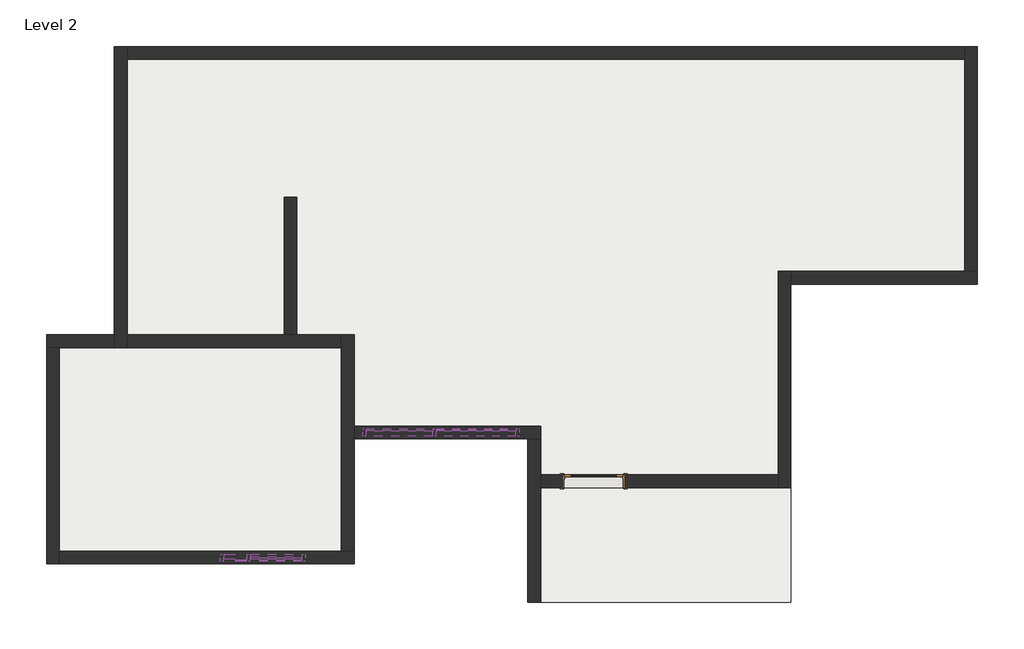
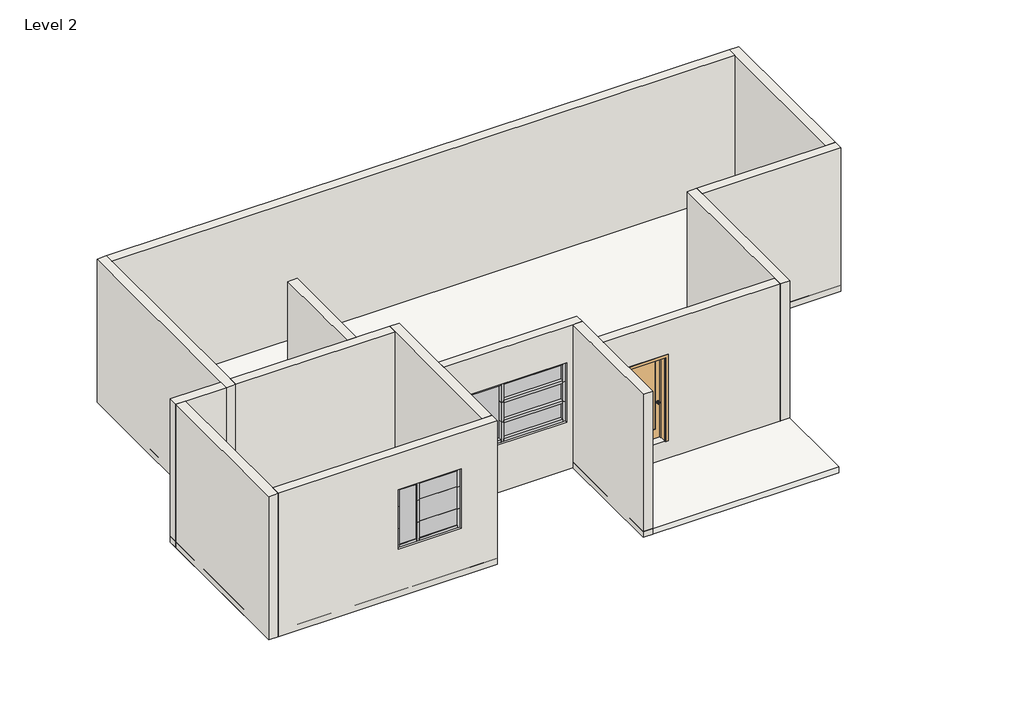
# One storey: 30 members, 14 walls, 8 plates, 1 door, 1 roof.
"""IFC4 building model written with IfcOpenShell, lengths in millimetres."""

from ifc_helpers import new_model, si_unit, frame, origin, place, context, project, spatial, polyline, outline, extrude, faceted_brep, transform, mapped, element, save
from components import door_0f538abb, member_df2e51ae, member_dc106669, member_ff82125d, member_323df77c, member_bc554fa6, member_86d06fe4, member_50cacee6, member_7fd687a9, member_26d67f61, member_e9c7f4a4, member_90750a43, member_6df10a9f, system_panel_glazed_08f033f8, system_panel_glazed_aa4e1581, system_panel_glazed_b16bc715, system_panel_glazed_e5754967, system_panel_glazed_03bb9a0f, system_panel_glazed_a826d7bb

model = new_model("IFC4")

# Units and contexts
model_context = context("Model", 3, world=origin())
ifc_project = project(units=[si_unit("LENGTHUNIT", "METRE", prefix="MILLI")], contexts=[model_context])

# Site, building, storey
site = spatial("IfcSite", under=ifc_project)
building = spatial("IfcBuilding", under=site)
storey = spatial("IfcBuildingStorey", under=building, Name="Level 2", Elevation=3048.0)

# Door
placement = place(None, origin())
door_shape = door_0f538abb(model_context)
element("IfcDoor", 1, ObjectType="Door-Interior-Single-1_Panel-Wood : 42\" x 84\"", at=placement, inside=storey, context=model_context, shape_type="MappedRepresentation", body=[
    mapped(door_shape, transform((-1951.8981007, 5916.5450124, 3657.6), x_axis=(-1.0, 0.0, 0.0), y_axis=(0.0, -1.0, 0.0), z_axis=(0.0, 0.0, 1.0))),
])

# Members
member_shape = member_df2e51ae(model_context)
element("IfcMember", 2, ObjectType="Rectangular Mullion : 1\" Square", at=placement, inside=storey, context=model_context, shape_type="MappedRepresentation", body=[
    mapped(member_shape, transform((-8117.7481007, 4541.7700124, 5308.6), x_axis=(0.0, 0.0, 1.0), y_axis=(0.0, 1.0, 0.0), z_axis=(-1.0, 0.0, 0.0))),
])
element("IfcMember", 3, ObjectType="Rectangular Mullion : 1\" Square", at=placement, inside=storey, context=model_context, shape_type="MappedRepresentation", body=[
    mapped(member_shape, transform((-8117.7481007, 4541.7700124, 4749.8), x_axis=(0.0, 0.0, 1.0), y_axis=(0.0, 1.0, 0.0), z_axis=(-1.0, 0.0, 0.0))),
])
member_2_shape = member_dc106669(model_context)
element("IfcMember", 4, ObjectType="Rectangular Mullion : 2.5\" x 5\" rectangular", at=placement, inside=storey, context=model_context, shape_type="MappedRepresentation", body=[
    mapped(member_2_shape, transform((-8593.9981007, 4541.7700124, 5791.2), x_axis=(0.0, 0.0, 1.0), y_axis=(0.0, 1.0, 0.0), z_axis=(-1.0, 0.0, 0.0))),
])
member_3_shape = member_ff82125d(model_context)
element("IfcMember", 5, ObjectType="Rectangular Mullion : 2.5\" x 5\" rectangular", at=placement, inside=storey, context=model_context, shape_type="MappedRepresentation", body=[
    mapped(member_3_shape, transform((-7196.9981007, 4541.7700124, 4267.2), x_axis=(0.0, 0.0, -1.0), y_axis=(0.0, 1.0, 0.0), z_axis=(1.0, 0.0, 0.0))),
])
member_4_shape = member_323df77c(model_context)
element("IfcMember", 6, ObjectType="Rectangular Mullion : 2.5\" x 5\" rectangular", at=placement, inside=storey, context=model_context, shape_type="MappedRepresentation", body=[
    mapped(member_4_shape, transform((-8149.4981007, 4541.7700124, 4267.2), x_axis=(-1.0, 0.0, 0.0), y_axis=(0.0, 1.0, 0.0), z_axis=(0.0, 0.0, -1.0))),
])
element("IfcMember", 7, ObjectType="Rectangular Mullion : 2.5\" x 5\" rectangular", at=placement, inside=storey, context=model_context, shape_type="MappedRepresentation", body=[
    mapped(member_2_shape, transform((-8181.2481007, 4541.7700124, 4267.2), x_axis=(0.0, 0.0, -1.0), y_axis=(0.0, 1.0, 0.0), z_axis=(1.0, 0.0, 0.0))),
])
element("IfcMember", 8, ObjectType="Rectangular Mullion : 2.5\" x 5\" rectangular", at=placement, inside=storey, context=model_context, shape_type="MappedRepresentation", body=[
    mapped(member_3_shape, transform((-8117.7481007, 4541.7700124, 5791.2), x_axis=(0.0, 0.0, 1.0), y_axis=(0.0, 1.0, 0.0), z_axis=(-1.0, 0.0, 0.0))),
])
member_5_shape = member_bc554fa6(model_context)
element("IfcMember", 9, ObjectType="Rectangular Mullion : 2.5\" x 5\" rectangular", at=placement, inside=storey, context=model_context, shape_type="MappedRepresentation", body=[
    mapped(member_5_shape, transform((-8149.4981007, 4541.7700124, 4749.8), x_axis=(-1.0, 0.0, 0.0), y_axis=(0.0, 1.0, 0.0), z_axis=(0.0, 0.0, -1.0))),
])
element("IfcMember", 10, ObjectType="Rectangular Mullion : 2.5\" x 5\" rectangular", at=placement, inside=storey, context=model_context, shape_type="MappedRepresentation", body=[
    mapped(member_4_shape, transform((-8149.4981007, 4541.7700124, 5308.6), x_axis=(-1.0, 0.0, 0.0), y_axis=(0.0, 1.0, 0.0), z_axis=(0.0, 0.0, -1.0))),
])
member_6_shape = member_86d06fe4(model_context)
element("IfcMember", 11, ObjectType="Rectangular Mullion : 2.5\" x 5\" rectangular", at=placement, inside=storey, context=model_context, shape_type="MappedRepresentation", body=[
    mapped(member_6_shape, transform((-7133.4981007, 4541.7700124, 5791.2), x_axis=(1.0, 0.0, 0.0), y_axis=(0.0, 1.0, 0.0), z_axis=(0.0, 0.0, 1.0))),
])
element("IfcMember", 12, ObjectType="Rectangular Mullion : 2.5\" x 5\" rectangular", at=placement, inside=storey, context=model_context, shape_type="MappedRepresentation", body=[
    mapped(member_6_shape, transform((-8657.4981007, 4541.7700124, 4267.2), x_axis=(-1.0, 0.0, 0.0), y_axis=(0.0, 1.0, 0.0), z_axis=(0.0, 0.0, -1.0))),
])
member_7_shape = member_50cacee6(model_context)
element("IfcMember", 13, ObjectType="Rectangular Mullion : 2.5\" x 5\" rectangular", at=placement, inside=storey, context=model_context, shape_type="MappedRepresentation", body=[
    mapped(member_7_shape, transform((-8657.4981007, 4541.7700124, 4749.8), x_axis=(-1.0, 0.0, 0.0), y_axis=(0.0, 1.0, 0.0), z_axis=(0.0, 0.0, -1.0))),
])
element("IfcMember", 14, ObjectType="Rectangular Mullion : 2.5\" x 5\" rectangular", at=placement, inside=storey, context=model_context, shape_type="MappedRepresentation", body=[
    mapped(member_6_shape, transform((-8657.4981007, 4541.7700124, 5308.6), x_axis=(-1.0, 0.0, 0.0), y_axis=(0.0, 1.0, 0.0), z_axis=(0.0, 0.0, -1.0))),
])
element("IfcMember", 15, ObjectType="Rectangular Mullion : 2.5\" x 5\" rectangular", at=placement, inside=storey, context=model_context, shape_type="MappedRepresentation", body=[
    mapped(member_6_shape, transform((-7133.4981007, 4541.7700124, 4749.8), x_axis=(1.0, 0.0, 0.0), y_axis=(0.0, 1.0, 0.0), z_axis=(0.0, 0.0, 1.0))),
])
element("IfcMember", 16, ObjectType="Rectangular Mullion : 2.5\" x 5\" rectangular", at=placement, inside=storey, context=model_context, shape_type="MappedRepresentation", body=[
    mapped(member_7_shape, transform((-7133.4981007, 4541.7700124, 5308.6), x_axis=(1.0, 0.0, 0.0), y_axis=(0.0, 1.0, 0.0), z_axis=(0.0, 0.0, 1.0))),
])
member_8_shape = member_7fd687a9(model_context)
element("IfcMember", 17, ObjectType="Rectangular Mullion : 2.5\" x 5\" rectangular", at=placement, inside=storey, context=model_context, shape_type="MappedRepresentation", body=[
    mapped(member_8_shape, transform((-6104.7981007, 6789.6700124, 5791.2), x_axis=(-1.0, 0.0, 0.0), y_axis=(0.0, -1.0, 0.0), z_axis=(0.0, 0.0, 1.0))),
])
element("IfcMember", 18, ObjectType="Rectangular Mullion : 2.5\" x 5\" rectangular", at=placement, inside=storey, context=model_context, shape_type="MappedRepresentation", body=[
    mapped(member_8_shape, transform((-6104.7981007, 6789.6700124, 5283.2), x_axis=(-1.0, 0.0, 0.0), y_axis=(0.0, -1.0, 0.0), z_axis=(0.0, 0.0, 1.0))),
])
element("IfcMember", 19, ObjectType="Rectangular Mullion : 2.5\" x 5\" rectangular", at=placement, inside=storey, context=model_context, shape_type="MappedRepresentation", body=[
    mapped(member_8_shape, transform((-6104.7981007, 6789.6700124, 4775.2), x_axis=(-1.0, 0.0, 0.0), y_axis=(0.0, -1.0, 0.0), z_axis=(0.0, 0.0, 1.0))),
])
member_9_shape = member_26d67f61(model_context)
element("IfcMember", 20, ObjectType="Rectangular Mullion : 2.5\" x 5\" rectangular", at=placement, inside=storey, context=model_context, shape_type="MappedRepresentation", body=[
    mapped(member_9_shape, transform((-3348.8981007, 6789.6700124, 5791.2), x_axis=(0.0, 0.0, 1.0), y_axis=(0.0, -1.0, 0.0), z_axis=(1.0, 0.0, 0.0))),
])
member_10_shape = member_e9c7f4a4(model_context)
element("IfcMember", 21, ObjectType="Rectangular Mullion : 2.5\" x 5\" rectangular", at=placement, inside=storey, context=model_context, shape_type="MappedRepresentation", body=[
    mapped(member_10_shape, transform((-6041.2981007, 6789.6700124, 4267.2), x_axis=(0.0, 0.0, -1.0), y_axis=(0.0, -1.0, 0.0), z_axis=(-1.0, 0.0, 0.0))),
])
element("IfcMember", 22, ObjectType="Rectangular Mullion : 2.5\" x 5\" rectangular", at=placement, inside=storey, context=model_context, shape_type="MappedRepresentation", body=[
    mapped(member_10_shape, transform((-4841.1481007, 6789.6700124, 5791.2), x_axis=(0.0, 0.0, 1.0), y_axis=(0.0, -1.0, 0.0), z_axis=(1.0, 0.0, 0.0))),
])
element("IfcMember", 23, ObjectType="Rectangular Mullion : 2.5\" x 5\" rectangular", at=placement, inside=storey, context=model_context, shape_type="MappedRepresentation", body=[
    mapped(member_9_shape, transform((-4777.6481007, 6789.6700124, 4267.2), x_axis=(0.0, 0.0, -1.0), y_axis=(0.0, -1.0, 0.0), z_axis=(-1.0, 0.0, 0.0))),
])
member_11_shape = member_90750a43(model_context)
element("IfcMember", 24, ObjectType="Rectangular Mullion : 2.5\" x 5\" rectangular", at=placement, inside=storey, context=model_context, shape_type="MappedRepresentation", body=[
    mapped(member_11_shape, transform((-4809.3981007, 6789.6700124, 4267.2), x_axis=(1.0, 0.0, 0.0), y_axis=(0.0, -1.0, 0.0), z_axis=(0.0, 0.0, -1.0))),
])
member_12_shape = member_6df10a9f(model_context)
element("IfcMember", 25, ObjectType="Rectangular Mullion : 2.5\" x 5\" rectangular", at=placement, inside=storey, context=model_context, shape_type="MappedRepresentation", body=[
    mapped(member_12_shape, transform((-3348.8981007, 6789.6700124, 5283.2), x_axis=(0.0, 0.0, 1.0), y_axis=(0.0, -1.0, 0.0), z_axis=(1.0, 0.0, 0.0))),
])
element("IfcMember", 26, ObjectType="Rectangular Mullion : 2.5\" x 5\" rectangular", at=placement, inside=storey, context=model_context, shape_type="MappedRepresentation", body=[
    mapped(member_12_shape, transform((-3348.8981007, 6789.6700124, 4775.2), x_axis=(0.0, 0.0, 1.0), y_axis=(0.0, -1.0, 0.0), z_axis=(1.0, 0.0, 0.0))),
])
element("IfcMember", 27, ObjectType="Rectangular Mullion : 2.5\" x 5\" rectangular", at=placement, inside=storey, context=model_context, shape_type="MappedRepresentation", body=[
    mapped(member_11_shape, transform((-4809.3981007, 6789.6700124, 5283.2), x_axis=(1.0, 0.0, 0.0), y_axis=(0.0, -1.0, 0.0), z_axis=(0.0, 0.0, -1.0))),
])
element("IfcMember", 28, ObjectType="Rectangular Mullion : 2.5\" x 5\" rectangular", at=placement, inside=storey, context=model_context, shape_type="MappedRepresentation", body=[
    mapped(member_11_shape, transform((-4809.3981007, 6789.6700124, 4775.2), x_axis=(1.0, 0.0, 0.0), y_axis=(0.0, -1.0, 0.0), z_axis=(0.0, 0.0, -1.0))),
])
element("IfcMember", 29, ObjectType="Rectangular Mullion : 2.5\" x 5\" rectangular", at=placement, inside=storey, context=model_context, shape_type="MappedRepresentation", body=[
    mapped(member_8_shape, transform((-3285.3981007, 6789.6700124, 4267.2), x_axis=(1.0, 0.0, 0.0), y_axis=(0.0, -1.0, 0.0), z_axis=(0.0, 0.0, -1.0))),
])
element("IfcMember", 30, ObjectType="Rectangular Mullion : 2.5\" x 5\" rectangular", at=placement, inside=storey, context=model_context, shape_type="MappedRepresentation", body=[
    mapped(member_8_shape, transform((-3285.3981007, 6789.6700124, 5283.2), x_axis=(1.0, 0.0, 0.0), y_axis=(0.0, -1.0, 0.0), z_axis=(0.0, 0.0, -1.0))),
])
element("IfcMember", 31, ObjectType="Rectangular Mullion : 2.5\" x 5\" rectangular", at=placement, inside=storey, context=model_context, shape_type="MappedRepresentation", body=[
    mapped(member_8_shape, transform((-3285.3981007, 6789.6700124, 4775.2), x_axis=(1.0, 0.0, 0.0), y_axis=(0.0, -1.0, 0.0), z_axis=(0.0, 0.0, -1.0))),
])

# Plates
system_panel_glazed_shape = system_panel_glazed_08f033f8(model_context)
element("IfcPlate", 32, ObjectType="System Panel : Glazed", at=placement, inside=storey, context=model_context, shape_type="MappedRepresentation", body=[
    mapped(system_panel_glazed_shape, transform((-7657.3731007, 4541.7700124, 4330.7), x_axis=(-1.0, 0.0, 0.0), y_axis=(0.0, -1.0, 0.0), z_axis=(0.0, 0.0, 1.0))),
])
element("IfcPlate", 33, ObjectType="System Panel : Glazed", at=placement, inside=storey, context=model_context, shape_type="MappedRepresentation", body=[
    mapped(system_panel_glazed_shape, transform((-7657.3731007, 4541.7700124, 5308.6), x_axis=(-1.0, 0.0, 0.0), y_axis=(0.0, -1.0, 0.0), z_axis=(0.0, 0.0, 1.0))),
])
system_panel_glazed_2_shape = system_panel_glazed_aa4e1581(model_context)
element("IfcPlate", 34, ObjectType="System Panel : Glazed", at=placement, inside=storey, context=model_context, shape_type="MappedRepresentation", body=[
    mapped(system_panel_glazed_2_shape, transform((-8387.6231007, 4541.7700124, 4330.7), x_axis=(-1.0, 0.0, 0.0), y_axis=(0.0, -1.0, 0.0), z_axis=(0.0, 0.0, 1.0))),
])
system_panel_glazed_3_shape = system_panel_glazed_b16bc715(model_context)
element("IfcPlate", 35, ObjectType="System Panel : Glazed", at=placement, inside=storey, context=model_context, shape_type="MappedRepresentation", body=[
    mapped(system_panel_glazed_3_shape, transform((-7657.3731007, 4541.7700124, 4749.8), x_axis=(-1.0, 0.0, 0.0), y_axis=(0.0, -1.0, 0.0), z_axis=(0.0, 0.0, 1.0))),
])
system_panel_glazed_4_shape = system_panel_glazed_e5754967(model_context)
element("IfcPlate", 36, ObjectType="System Panel : Glazed", at=placement, inside=storey, context=model_context, shape_type="MappedRepresentation", body=[
    mapped(system_panel_glazed_4_shape, transform((-5441.2231007, 6789.6700124, 4330.7), x_axis=(1.0, 0.0, 0.0), y_axis=(0.0, 1.0, 0.0), z_axis=(0.0, 0.0, 1.0))),
])
system_panel_glazed_5_shape = system_panel_glazed_03bb9a0f(model_context)
element("IfcPlate", 37, ObjectType="System Panel : Glazed", at=placement, inside=storey, context=model_context, shape_type="MappedRepresentation", body=[
    mapped(system_panel_glazed_5_shape, transform((-4063.2731007, 6789.6700124, 4330.7), x_axis=(1.0, 0.0, 0.0), y_axis=(0.0, 1.0, 0.0), z_axis=(0.0, 0.0, 1.0))),
])
element("IfcPlate", 38, ObjectType="System Panel : Glazed", at=placement, inside=storey, context=model_context, shape_type="MappedRepresentation", body=[
    mapped(system_panel_glazed_5_shape, transform((-4063.2731007, 6789.6700124, 5314.95), x_axis=(1.0, 0.0, 0.0), y_axis=(0.0, 1.0, 0.0), z_axis=(0.0, 0.0, 1.0))),
])
system_panel_glazed_6_shape = system_panel_glazed_a826d7bb(model_context)
element("IfcPlate", 39, ObjectType="System Panel : Glazed", at=placement, inside=storey, context=model_context, shape_type="MappedRepresentation", body=[
    mapped(system_panel_glazed_6_shape, transform((-4063.2731007, 6789.6700124, 4806.95), x_axis=(1.0, 0.0, 0.0), y_axis=(0.0, 1.0, 0.0), z_axis=(0.0, 0.0, 1.0))),
])

# Roof
element("IfcRoof", 40, ObjectType="6\" roof", at=placement, inside=storey, context=model_context, shape_type="SweptSolid", body=[
    extrude(outline(polyline([(-10562.4981007, 13723.8700124), (4944.2018993, 13723.8700124), (4944.2018993, 9456.6700124), (1591.4018993, 9456.6700124), (1591.4018993, 6300.0267693), (1591.4018993, 3741.6700124), (-3132.9981007, 3741.6700124), (-3132.9981007, 6675.3700124), (-6257.1981007, 6675.3700124), (-6257.1981007, 4427.4700124), (-11781.6981007, 4427.4700124), (-11781.6981007, 8542.2700124), (-10562.4981007, 8542.2700124), (-10562.4981007, 13723.8700124)])), frame((0.0, 0.0, 3048.0), z_axis=(0.0, 0.0, 1.0), x_axis=(1.0, 0.0, 0.0)), (0.0, 0.0, 1.0), 152.4),
])

# Walls
element("IfcWall", 41, ObjectType="9\" wall", at=placement, inside=storey, context=model_context, shape_type="Brep", body=[
    faceted_brep([(-10562.4981007, 13723.8700124, 3048.0), (-10562.4981007, 8542.2700124, 3048.0), (-10562.4981007, 8313.6700124, 3048.0), (-10562.4981007, 8313.6700124, 6705.6), (-10562.4981007, 8542.2700124, 6705.6), (-10562.4981007, 13723.8700124, 6705.6), (-10333.8981007, 13723.8700124, 3048.0), (-10333.8981007, 13723.8700124, 6705.6), (-10333.8981007, 13495.2700124, 6705.6), (-10333.8981007, 8542.2700124, 6705.6), (-10333.8981007, 8313.6700124, 6705.6), (-10333.8981007, 8313.6700124, 3048.0), (-10333.8981007, 8542.2700124, 3048.0), (-10333.8981007, 13495.2700124, 3048.0)], [[[0, 1, 2, 3, 4, 5]], [[6, 7, 8, 9, 10, 11, 12, 13]], [[2, 1, 0, 6, 13, 12, 11]], [[5, 4, 3, 10, 9, 8, 7]], [[3, 2, 11, 10]], [[0, 5, 7, 6]]]),
])
element("IfcWall", 42, ObjectType="9\" wall", at=placement, inside=storey, context=model_context, shape_type="Brep", body=[
    faceted_brep([(-10562.4981007, 8542.2700124, 3048.0), (-11781.6981007, 8542.2700124, 3048.0), (-11781.6981007, 8542.2700124, 6705.6), (-10562.4981007, 8542.2700124, 6705.6), (-10562.4981007, 8313.6700124, 3048.0), (-10562.4981007, 8313.6700124, 6705.6), (-11553.0981007, 8313.6700124, 6705.6), (-11781.6981007, 8313.6700124, 6705.6), (-11781.6981007, 8313.6700124, 3048.0), (-11553.0981007, 8313.6700124, 3048.0)], [[[0, 1, 2, 3]], [[4, 5, 6, 7, 8, 9]], [[1, 0, 4, 9, 8]], [[3, 2, 7, 6, 5]], [[0, 3, 5, 4]], [[2, 1, 8, 7]]]),
])
element("IfcWall", 43, ObjectType="9\" wall", at=placement, inside=storey, context=model_context, shape_type="Brep", body=[
    faceted_brep([(-11781.6981007, 8313.6700124, 3048.0), (-11781.6981007, 4427.4700124, 3048.0), (-11781.6981007, 4427.4700124, 6705.6), (-11781.6981007, 8313.6700124, 6705.6), (-11553.0981007, 8313.6700124, 3048.0), (-11553.0981007, 8313.6700124, 6705.6), (-11553.0981007, 4656.0700124, 6705.6), (-11553.0981007, 4427.4700124, 6705.6), (-11553.0981007, 4427.4700124, 3048.0), (-11553.0981007, 4656.0700124, 3048.0)], [[[0, 1, 2, 3]], [[4, 5, 6, 7, 8, 9]], [[1, 0, 4, 9, 8]], [[3, 2, 7, 6, 5]], [[0, 3, 5, 4]], [[2, 1, 8, 7]]]),
])
element("IfcWall", 44, ObjectType="9\" wall", at=placement, inside=storey, context=model_context, shape_type="Brep", body=[
    faceted_brep([(-11553.0981007, 4427.4700124, 3048.0), (-6257.1981007, 4427.4700124, 3048.0), (-6257.1981007, 4427.4700124, 6705.6), (-11553.0981007, 4427.4700124, 6705.6), (-7133.4981007, 4427.4700124, 5791.2), (-7133.4981007, 4427.4700124, 4267.2), (-8657.4981007, 4427.4700124, 4267.2), (-8657.4981007, 4427.4700124, 5791.2), (-6257.1981007, 4656.0700124, 3048.0), (-6485.7981007, 4656.0700124, 3048.0), (-11553.0981007, 4656.0700124, 3048.0), (-11553.0981007, 4656.0700124, 6705.6), (-6485.7981007, 4656.0700124, 6705.6), (-6257.1981007, 4656.0700124, 6705.6), (-7133.4981007, 4656.0700124, 4267.2), (-7133.4981007, 4656.0700124, 5791.2), (-8657.4981007, 4656.0700124, 5791.2), (-8657.4981007, 4656.0700124, 4267.2)], [[[0, 1, 2, 3], [4, 5, 6, 7]], [[8, 9, 10, 11, 12, 13], [14, 15, 16, 17]], [[1, 0, 10, 9, 8]], [[3, 2, 13, 12, 11]], [[0, 3, 11, 10]], [[2, 1, 8, 13]], [[14, 5, 4, 15]], [[15, 4, 7, 16]], [[16, 7, 6, 17]], [[5, 14, 17, 6]]]),
])
element("IfcWall", 45, ObjectType="9\" wall", at=placement, inside=storey, context=model_context, shape_type="Brep", body=[
    faceted_brep([(-6257.1981007, 4656.0700124, 3048.0), (-6257.1981007, 6675.3700124, 3048.0), (-6257.1981007, 6903.9700124, 3048.0), (-6257.1981007, 8542.2700124, 3048.0), (-6257.1981007, 8542.2700124, 6705.6), (-6257.1981007, 6903.9700124, 6705.6), (-6257.1981007, 6675.3700124, 6705.6), (-6257.1981007, 4656.0700124, 6705.6), (-6485.7981007, 4656.0700124, 3048.0), (-6485.7981007, 4656.0700124, 6705.6), (-6485.7981007, 8313.6700124, 6705.6), (-6485.7981007, 8542.2700124, 6705.6), (-6485.7981007, 8542.2700124, 3048.0), (-6485.7981007, 8313.6700124, 3048.0)], [[[0, 1, 2, 3, 4, 5, 6, 7]], [[8, 9, 10, 11, 12, 13]], [[3, 2, 1, 0, 8, 13, 12]], [[7, 6, 5, 4, 11, 10, 9]], [[0, 7, 9, 8]], [[4, 3, 12, 11]]]),
])
element("IfcWall", 46, ObjectType="9\" wall", at=placement, inside=storey, context=model_context, shape_type="Brep", body=[
    faceted_brep([(-10333.8981007, 8313.6700124, 3048.0), (-6485.7981007, 8313.6700124, 3048.0), (-6485.7981007, 8313.6700124, 6705.6), (-10333.8981007, 8313.6700124, 6705.6), (-10333.8981007, 8542.2700124, 3048.0), (-10333.8981007, 8542.2700124, 6705.6), (-7514.4981007, 8542.2700124, 6705.6), (-7285.8981007, 8542.2700124, 6705.6), (-6485.7981007, 8542.2700124, 6705.6), (-6485.7981007, 8542.2700124, 3048.0), (-7285.8981007, 8542.2700124, 3048.0), (-7514.4981007, 8542.2700124, 3048.0)], [[[0, 1, 2, 3]], [[4, 5, 6, 7, 8, 9, 10, 11]], [[1, 0, 4, 11, 10, 9]], [[3, 2, 8, 7, 6, 5]], [[0, 3, 5, 4]], [[2, 1, 9, 8]]]),
])
element("IfcWall", 47, ObjectType="9\" wall", at=placement, inside=storey, context=model_context, shape_type="SweptSolid", body=[
    extrude(outline(polyline([(-7285.8981007, 11018.7700124), (-7285.8981007, 8542.2700124), (-7514.4981007, 8542.2700124), (-7514.4981007, 11018.7700124), (-7285.8981007, 11018.7700124)])), frame((0.0, 0.0, 3048.0), z_axis=(0.0, 0.0, 1.0), x_axis=(1.0, 0.0, 0.0)), (0.0, 0.0, 1.0), 3657.6),
])
element("IfcWall", 48, ObjectType="9\" wall", at=placement, inside=storey, context=model_context, shape_type="Brep", body=[
    faceted_brep([(-6257.1981007, 6675.3700124, 3048.0), (-3132.9981007, 6675.3700124, 3048.0), (-2904.3981007, 6675.3700124, 3048.0), (-2904.3981007, 6675.3700124, 6705.6), (-3132.9981007, 6675.3700124, 6705.6), (-6257.1981007, 6675.3700124, 6705.6), (-6104.7981007, 6675.3700124, 4267.2), (-6104.7981007, 6675.3700124, 5791.2), (-3285.3981007, 6675.3700124, 5791.2), (-3285.3981007, 6675.3700124, 4267.2), (-2904.3981007, 6903.9700124, 3048.0), (-6257.1981007, 6903.9700124, 3048.0), (-6257.1981007, 6903.9700124, 6705.6), (-2904.3981007, 6903.9700124, 6705.6), (-6104.7981007, 6903.9700124, 5791.2), (-6104.7981007, 6903.9700124, 4267.2), (-3285.3981007, 6903.9700124, 4267.2), (-3285.3981007, 6903.9700124, 5791.2)], [[[0, 1, 2, 3, 4, 5], [6, 7, 8, 9]], [[10, 11, 12, 13], [14, 15, 16, 17]], [[2, 1, 0, 11, 10]], [[5, 4, 3, 13, 12]], [[0, 5, 12, 11]], [[3, 2, 10, 13]], [[6, 15, 14, 7]], [[7, 14, 17, 8]], [[8, 17, 16, 9]], [[15, 6, 9, 16]]]),
])
element("IfcWall", 49, ObjectType="9\" wall", at=placement, inside=storey, context=model_context, shape_type="Brep", body=[
    faceted_brep([(-3132.9981007, 6675.3700124, 3048.0), (-3132.9981007, 3741.6700124, 3048.0), (-3132.9981007, 3741.6700124, 6705.6), (-3132.9981007, 6675.3700124, 6705.6), (-2904.3981007, 6675.3700124, 3048.0), (-2904.3981007, 6675.3700124, 6705.6), (-2904.3981007, 6027.6700124, 6705.6), (-2904.3981007, 5799.0700124, 6705.6), (-2904.3981007, 3741.6700124, 6705.6), (-2904.3981007, 3741.6700124, 3048.0), (-2904.3981007, 5799.0700124, 3048.0), (-2904.3981007, 6027.6700124, 3048.0)], [[[0, 1, 2, 3]], [[4, 5, 6, 7, 8, 9, 10, 11]], [[1, 0, 4, 11, 10, 9]], [[2, 1, 9, 8]], [[3, 2, 8, 7, 6, 5]], [[0, 3, 5, 4]]]),
])
element("IfcWall", 50, ObjectType="9\" wall", at=placement, inside=storey, context=model_context, shape_type="Brep", body=[
    faceted_brep([(1591.4018993, 5799.0700124, 3048.0), (1591.4018993, 9456.6700124, 3048.0), (1591.4018993, 9685.2700124, 3048.0), (1591.4018993, 9685.2700124, 6705.6), (1591.4018993, 9456.6700124, 6705.6), (1591.4018993, 5799.0700124, 6705.6), (1362.8018993, 5799.0700124, 3048.0), (1362.8018993, 5799.0700124, 6705.6), (1362.8018993, 6027.6700124, 6705.6), (1362.8018993, 9685.2700124, 6705.6), (1362.8018993, 9685.2700124, 3048.0), (1362.8018993, 6027.6700124, 3048.0)], [[[0, 1, 2, 3, 4, 5]], [[6, 7, 8, 9, 10, 11]], [[2, 1, 0, 6, 11, 10]], [[5, 4, 3, 9, 8, 7]], [[3, 2, 10, 9]], [[0, 5, 7, 6]]]),
])
element("IfcWall", 51, ObjectType="9\" wall", at=placement, inside=storey, context=model_context, shape_type="Brep", body=[
    faceted_brep([(1591.4018993, 9456.6700124, 3048.0), (4944.2018993, 9456.6700124, 3048.0), (4944.2018993, 9456.6700124, 6705.6), (1591.4018993, 9456.6700124, 6705.6), (1591.4018993, 9685.2700124, 3048.0), (1591.4018993, 9685.2700124, 6705.6), (4715.6018993, 9685.2700124, 6705.6), (4944.2018993, 9685.2700124, 6705.6), (4944.2018993, 9685.2700124, 3048.0), (4715.6018993, 9685.2700124, 3048.0)], [[[0, 1, 2, 3]], [[4, 5, 6, 7, 8, 9]], [[1, 0, 4, 9, 8]], [[3, 2, 7, 6, 5]], [[0, 3, 5, 4]], [[2, 1, 8, 7]]]),
])
element("IfcWall", 52, ObjectType="9\" wall", at=placement, inside=storey, context=model_context, shape_type="Brep", body=[
    faceted_brep([(4944.2018993, 9685.2700124, 3048.0), (4944.2018993, 13723.8700124, 3048.0), (4944.2018993, 13723.8700124, 6705.6), (4944.2018993, 9685.2700124, 6705.6), (4715.6018993, 9685.2700124, 3048.0), (4715.6018993, 9685.2700124, 6705.6), (4715.6018993, 13495.2700124, 6705.6), (4715.6018993, 13723.8700124, 6705.6), (4715.6018993, 13723.8700124, 3048.0), (4715.6018993, 13495.2700124, 3048.0)], [[[0, 1, 2, 3]], [[4, 5, 6, 7, 8, 9]], [[1, 0, 4, 9, 8]], [[3, 2, 7, 6, 5]], [[0, 3, 5, 4]], [[2, 1, 8, 7]]]),
])
element("IfcWall", 53, ObjectType="9\" wall", at=placement, inside=storey, context=model_context, shape_type="SweptSolid", body=[
    extrude(outline(polyline([(-10333.8981007, 13723.8700124), (4715.6018993, 13723.8700124), (4715.6018993, 13495.2700124), (-10333.8981007, 13495.2700124), (-10333.8981007, 13723.8700124)])), frame((0.0, 0.0, 3048.0), z_axis=(0.0, 0.0, 1.0), x_axis=(1.0, 0.0, 0.0)), (0.0, 0.0, 1.0), 3657.6),
])
element("IfcWall", 54, ObjectType="9\" wall", at=placement, inside=storey, context=model_context, shape_type="SweptSolid", body=[
    extrude(outline(polyline([(3048.0, -2904.3981007), (3048.0, 1362.8018993), (6705.6, 1362.8018993), (6705.6, -2904.3981007), (3048.0, -2904.3981007)]), holes=[polyline([(3657.6, -2510.6981007), (5816.6, -2510.6981007), (5816.6, -1393.0981007), (3657.6, -1393.0981007), (3657.6, -2510.6981007)])]), frame((0.0, 5799.0700124, 0.0), z_axis=(0.0, 1.0, 0.0), x_axis=(0.0, 0.0, 1.0)), (0.0, 0.0, 1.0), 228.6),
])

save(model, "model.ifc")

# Revit data of these elements
# Type "Door-Interior-Single-1_Panel-Wood : 42\" x 84\""
#   Type Mark = "9"
#   Assembly Code = "C1020300"
#   Analytic Construction = "Wooden"
#   Top Rail = 0' - 4 11/16"
#   Thickness = 0' - 1 3/8"
#   Thermal Resistance (R) = 2.5876 (h·ft²·°F)/BTU
#   Swing Angle [instance default] = 90.00°
#   Stiles = 0' - 4 3/4"
#   Rough Width = 3' - 8"
#   Rough Height = 7' - 1"
#   Height = 7' - 0"
#   Width = 3' - 6"
#   Heat Transfer Coefficient (U) = 0.3865 BTU/(h·ft²·°F)
#   Bottom Rail = 0' - 9 1/8"
#   Trim Material = Cherry
#   Panel Material = Cherry
#   Frame Material = Cherry
#   Door Handle Material = Aluminum
#   Visual Light Transmittance = 0
#   Solar Heat Gain Coefficient = 0
#   Wall Closure = (empty or 0)
#   Function = (empty or 0)
# Type "Rectangular Mullion : 1\" Square"
#   built-in parameter 1007304 = 0.0833333 (stored number, unit not read)
#   built-in parameter 1007301 = 0.0416667 (stored number, unit not read)
#   built-in parameter 1007300 = 0.0416667 (stored number, unit not read)
# Type "Rectangular Mullion : 2.5\" x 5\" rectangular"
#   built-in parameter 1007304 = 0.416667 (stored number, unit not read)
#   built-in parameter 1007301 = 0.104167 (stored number, unit not read)
#   built-in parameter 1007300 = 0.104167 (stored number, unit not read)
# Type "System Panel : Glazed"
#   Construction Type Id = "GSP4R"
#   Analytic Construction = "1/8 in Pilkington single glazing"
#   Visual Light Transmittance = 0.9
#   Solar Heat Gain Coefficient = 0.86
#   Heat Transfer Coefficient (U) = 1.18115 BTU/(h·ft²·°F)
#   Define Thermal Properties by = 1
# Type "6\" roof"
#   Assembly Code = "B1020"
#   Layers, outside or top first: 0' - 6" no material (function 1)
# Type "9\" wall"
#   Assembly Code = "B2010"
#   Layers, outside or top first: 0' - 9" no material (function 1)
# Element 1 (IfcDoor, "Door-Interior-Single-1_Panel-Wood : 42\" x 84\"")
#   Swing Angle = 90.00°
#   Phase Created = New Construction
#   Materials on its faces: "Cherry", "Aluminum"
# Elements 2, 3 (IfcMember, "Rectangular Mullion : 1\" Square")
#   Phase Created = New Construction
#   Materials on its faces: "Rectangle 1 sq"
# Elements 4, 5, 6, 7, 8, 9, 10, 11, 12, 13, 14, 15, 16, 17, 18, 19, 20, 21, 22, 23, 24, 25, 26, 27, 28, 29, 30, 31 (IfcMember, "Rectangular Mullion : 2.5\" x 5\" rectangular")
#   Phase Created = New Construction
#   Materials on its faces: "Rectangle 1 sq"
# Elements 32, 33, 34, 35, 36, 37, 38, 39 (IfcPlate, "System Panel : Glazed")
#   Phase Created = New Construction
#   Materials on its faces: "Glass"
# Element 40 (IfcRoof, "6\" roof")
#   built-in parameter 1001705 = 10.5 (stored number, unit not read)
#   built-in parameter 1001710 = 33615
#   Phase Created = New Construction
#   Materials on its faces: "Default Roof"
# Elements 41, 42, 43, 44, 45, 46, 47, 48, 49, 50, 51, 52, 53, 54 (IfcWall, "9\" wall")
#   Top Offset = 1' - 6"
#   Base Offset = 0' - 0"
#   wall height = 12' - 0"
#   Phase Created = New Construction
#   Base Constraint = Level 2
#   Top Constraint = Level 4
#   Materials on its faces: "Default Wall"
# Materials
#   "Cherry": class "Wood", colour RGB 226 177 128, transparency 0, Description = "Prunus Serotina", Cost = 0
#   "Aluminum": class "Metal", colour RGB 247 247 247, transparency 0, Description = "Aluminum 6061", Cost = 0
#   "Rectangle 1 sq": class "Generic", colour RGB 120 120 120, transparency 0, Cost = 0
#   "Glass": class "Glass", colour RGB 0 128 192, transparency 0.75, Description = "Soda Lime Glass", Cost = 0
#   "Default Roof": colour RGB 88 101 114, transparency 0, Cost = 0
#   "Default Wall": colour RGB 128 128 128, transparency 0, Cost = 0
